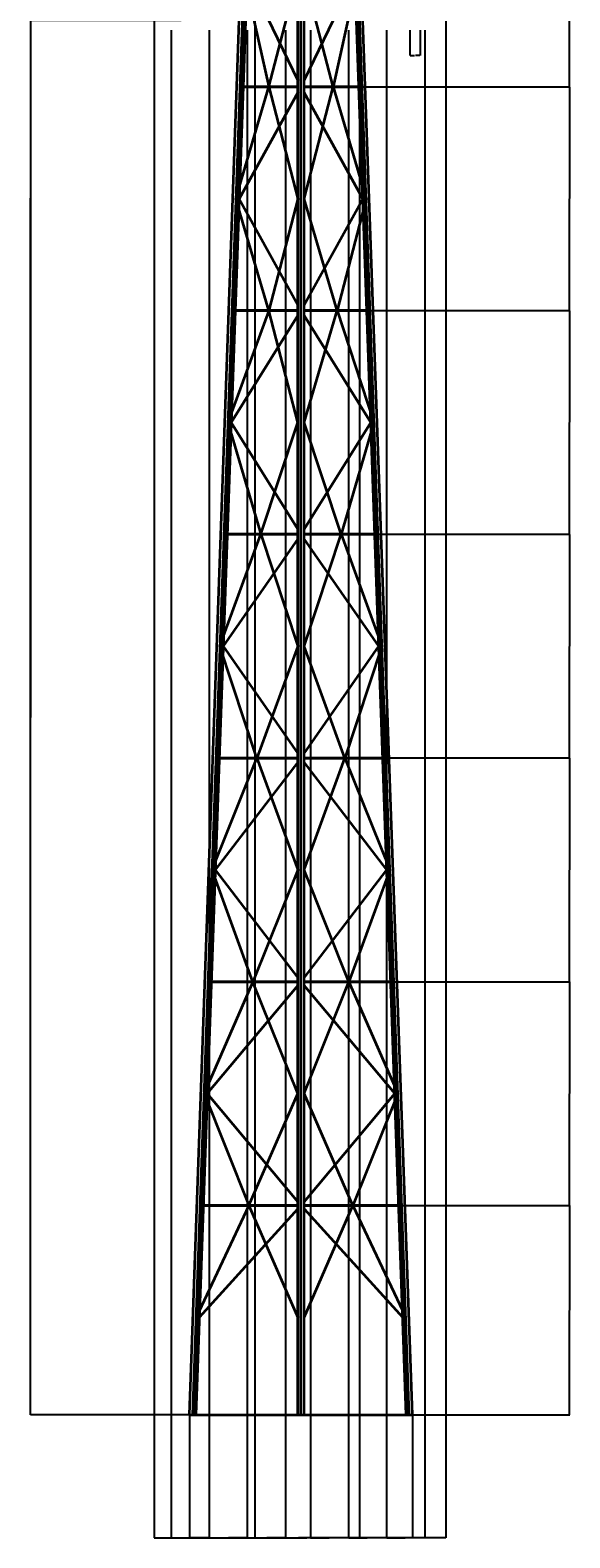
# Model space of a CAD drawing. Units: inches. Extents: x 3780 to 4301, y 1637 to 4224.
# Tile 1 of 8: x 3780 to 4301, y 1637 to 3092. Entities that reach past the tile are written whole.
import ezdxf

# ---------------------------------------------------------------- set-up
doc = ezdxf.new("R2010")
doc.units = ezdxf.units.IN
doc.layers.add('A-ANNO-DIMS', color=2, linetype='Continuous', lineweight=18)
doc.layers.add('S-TOWR', color=7, linetype='Continuous', lineweight=35)
doc.styles.get("Standard").update_dxf_attribs({"font": 'arial.ttf'})
doc.dimstyles.get("Standard").update_dxf_attribs({"dimtxt": 0.18, "dimasz": 0.18, "dimexe": 0.18, "dimexo": 0.0625, "dimgap": 0.09, "dimtad": 0, "dimtih": 1, "dimtoh": 1, "dimdec": 4, "dimzin": 0, "dimdsep": 46, "dimtxsty": 'Standard', "dimcen": 0.09, "dimadec": 0, "dimazin": 0, "dimtfac": 1, "dimtdec": 4, "dimtofl": 0, "dimtmove": 0, "dimatfit": 3, "dimfxl": 1, "dimtolj": 1, "dimtzin": 0, "dimarcsym": 0})

# ---------------------------------------------------------------- blocks, each defined once
blk = doc.blocks.new('*D10')
at = {"layer": 'A-ANNO-DIMS', "color": 0, "lineweight": -2, "transparency": 16777216}
for p, q in [((4146.7, 3092.2), (4146.7, 3067.7)), ((4156.5, 3092.2), (4156.5, 3067.7)), ((4146.9, 3067.9), (4151.1, 3067.9)), ((4156.3, 3067.9), (4152.1, 3067.9))]:
    blk.add_line(p, q, dxfattribs=at)
at = {"layer": 'A-ANNO-DIMS', "color": 0, "transparency": 16777216}
for points in [[(4146.9, 3067.9), (4146.9, 3067.9), (4146.7, 3067.9)], [(4156.3, 3067.9), (4156.3, 3067.9), (4156.5, 3067.9)]]:
    blk.add_solid(points, dxfattribs=at)
at = {"layer": 'Defpoints', "color": 0, "transparency": 16777216}
for p in [(4146.7, 3092.2), (4156.5, 3092.2), (4156.5, 3067.9)]:
    blk.add_point(p, dxfattribs=at)
at = {"layer": 'A-ANNO-DIMS', "color": 0, "transparency": 16777216, "insert": (4151.6, 3067.9), "char_height": 0.18, "attachment_point": 5}
blk.add_mtext('\\A1;10 TYP.', dxfattribs=at)
blk = doc.blocks.new('*D11')
at = {"layer": 'A-ANNO-DIMS', "color": 0, "lineweight": -2, "transparency": 16777216}
for p, q in [((3916.2, 4105.3), (3780.7, 4105.3)), ((3780.8, 4105.1), (3780.8, 2930.4)), ((3780.8, 1755.4), (3780.8, 2930.1)), ((3934.1, 1755.2), (3780.7, 1755.2))]:
    blk.add_line(p, q, dxfattribs=at)
at = {"layer": 'A-ANNO-DIMS', "color": 0, "transparency": 16777216}
for points in [[(3780.8, 4105.1), (3780.9, 4105.1), (3780.8, 4105.3)], [(3780.8, 1755.4), (3780.9, 1755.4), (3780.8, 1755.2)]]:
    blk.add_solid(points, dxfattribs=at)
at = {"layer": 'Defpoints', "color": 0, "transparency": 16777216}
for p in [(3780.8, 4105.3), (3916.3, 4105.3), (3934.2, 1755.2)]:
    blk.add_point(p, dxfattribs=at)
at = {"layer": 'A-ANNO-DIMS', "color": 0, "transparency": 16777216, "insert": (3780.8, 2930.3), "char_height": 0.18, "attachment_point": 5}
blk.add_mtext('\\A1;2350', dxfattribs=at)
blk = doc.blocks.new('*D12')
at = {"layer": 'A-ANNO-DIMS', "color": 0, "lineweight": -2, "transparency": 16777216}
for p, q in [((3934.2, 1755.2), (3934.2, 1636.6)), ((4149.2, 1755.2), (4149.2, 1636.6)), ((3934.3, 1636.7), (4041.4, 1636.7)), ((4149, 1636.7), (4042, 1636.7))]:
    blk.add_line(p, q, dxfattribs=at)
at = {"layer": 'A-ANNO-DIMS', "color": 0, "transparency": 16777216}
for points in [[(3934.3, 1636.8), (3934.3, 1636.7), (3934.2, 1636.7)], [(4149, 1636.8), (4149, 1636.7), (4149.2, 1636.7)]]:
    blk.add_solid(points, dxfattribs=at)
at = {"layer": 'Defpoints', "color": 0, "transparency": 16777216}
for p in [(3934.2, 1755.2), (4149.2, 1755.2), (4149.2, 1636.7)]:
    blk.add_point(p, dxfattribs=at)
at = {"layer": 'A-ANNO-DIMS', "color": 0, "transparency": 16777216, "insert": (4041.7, 1636.7), "char_height": 0.18, "attachment_point": 5}
blk.add_mtext('\\A1;215', dxfattribs=at)
blk = doc.blocks.new('*D13')
at = {"layer": 'A-ANNO-DIMS', "color": 0, "lineweight": -2, "transparency": 16777216}
for p, q in [((4044.7, 1957.5), (4300.9, 1957.5)), ((4300.7, 1957.3), (4300.7, 1856.5)), ((4300.7, 1755.4), (4300.7, 1856.2)), ((4044.7, 1755.2), (4300.9, 1755.2))]:
    blk.add_line(p, q, dxfattribs=at)
at = {"layer": 'A-ANNO-DIMS', "color": 0, "transparency": 16777216}
for points in [[(4300.7, 1957.3), (4300.7, 1957.3), (4300.7, 1957.5)], [(4300.7, 1755.4), (4300.7, 1755.4), (4300.7, 1755.2)]]:
    blk.add_solid(points, dxfattribs=at)
at = {"layer": 'Defpoints', "color": 0, "transparency": 16777216}
for p in [(4044.7, 1957.5), (4300.7, 1957.5), (4044.7, 1755.2)]:
    blk.add_point(p, dxfattribs=at)
at = {"layer": 'A-ANNO-DIMS', "color": 0, "transparency": 16777216, "insert": (4300.7, 1856.4), "char_height": 0.18, "attachment_point": 5}
blk.add_mtext('\\A1;202.2', dxfattribs=at)
blk = doc.blocks.new('*D14')
at = {"layer": 'A-ANNO-DIMS', "color": 0, "lineweight": -2, "transparency": 16777216}
for p, q in [((4044.7, 2173.5), (4300.9, 2173.5)), ((4300.7, 2173.3), (4300.7, 2065.6)), ((4300.7, 1957.6), (4300.7, 2065.3)), ((4044.7, 1957.5), (4300.9, 1957.5))]:
    blk.add_line(p, q, dxfattribs=at)
at = {"layer": 'A-ANNO-DIMS', "color": 0, "transparency": 16777216}
for points in [[(4300.7, 2173.3), (4300.7, 2173.3), (4300.7, 2173.5)], [(4300.7, 1957.6), (4300.7, 1957.6), (4300.7, 1957.5)]]:
    blk.add_solid(points, dxfattribs=at)
at = {"layer": 'Defpoints', "color": 0, "transparency": 16777216}
for p in [(4044.7, 2173.5), (4300.7, 2173.5), (4044.7, 1957.5)]:
    blk.add_point(p, dxfattribs=at)
at = {"layer": 'A-ANNO-DIMS', "color": 0, "transparency": 16777216, "insert": (4300.7, 2065.5), "char_height": 0.18, "attachment_point": 5}
blk.add_mtext('\\A1;216', dxfattribs=at)
blk = doc.blocks.new('*D15')
at = {"layer": 'A-ANNO-DIMS', "color": 0, "lineweight": -2, "transparency": 16777216}
for p, q in [((4044.7, 2389.5), (4300.9, 2389.5)), ((4300.7, 2389.3), (4300.7, 2281.6)), ((4300.7, 2173.6), (4300.7, 2281.3)), ((4044.7, 2173.5), (4300.9, 2173.5))]:
    blk.add_line(p, q, dxfattribs=at)
at = {"layer": 'A-ANNO-DIMS', "color": 0, "transparency": 16777216}
for points in [[(4300.7, 2389.3), (4300.7, 2389.3), (4300.7, 2389.5)], [(4300.7, 2173.6), (4300.7, 2173.6), (4300.7, 2173.5)]]:
    blk.add_solid(points, dxfattribs=at)
at = {"layer": 'Defpoints', "color": 0, "transparency": 16777216}
for p in [(4044.7, 2389.5), (4300.7, 2389.5), (4044.7, 2173.5)]:
    blk.add_point(p, dxfattribs=at)
at = {"layer": 'A-ANNO-DIMS', "color": 0, "transparency": 16777216, "insert": (4300.7, 2281.5), "char_height": 0.18, "attachment_point": 5}
blk.add_mtext('\\A1;216', dxfattribs=at)
blk = doc.blocks.new('*D16')
at = {"layer": 'A-ANNO-DIMS', "color": 0, "lineweight": -2, "transparency": 16777216}
for p, q in [((4044.7, 2605.5), (4300.9, 2605.5)), ((4300.7, 2605.3), (4300.7, 2497.6)), ((4300.7, 2389.6), (4300.7, 2497.3)), ((4044.7, 2389.5), (4300.9, 2389.5))]:
    blk.add_line(p, q, dxfattribs=at)
at = {"layer": 'A-ANNO-DIMS', "color": 0, "transparency": 16777216}
for points in [[(4300.7, 2605.3), (4300.7, 2605.3), (4300.7, 2605.5)], [(4300.7, 2389.6), (4300.7, 2389.6), (4300.7, 2389.5)]]:
    blk.add_solid(points, dxfattribs=at)
at = {"layer": 'Defpoints', "color": 0, "transparency": 16777216}
for p in [(4044.7, 2605.5), (4300.7, 2605.5), (4044.7, 2389.5)]:
    blk.add_point(p, dxfattribs=at)
at = {"layer": 'A-ANNO-DIMS', "color": 0, "transparency": 16777216, "insert": (4300.7, 2497.5), "char_height": 0.18, "attachment_point": 5}
blk.add_mtext('\\A1;216', dxfattribs=at)
blk = doc.blocks.new('*D17')
at = {"layer": 'A-ANNO-DIMS', "color": 0, "lineweight": -2, "transparency": 16777216}
for p, q in [((4044.7, 2821.5), (4300.9, 2821.5)), ((4300.7, 2821.3), (4300.7, 2713.6)), ((4300.7, 2605.6), (4300.7, 2713.3)), ((4044.7, 2605.5), (4300.9, 2605.5))]:
    blk.add_line(p, q, dxfattribs=at)
at = {"layer": 'A-ANNO-DIMS', "color": 0, "transparency": 16777216}
for points in [[(4300.7, 2821.3), (4300.7, 2821.3), (4300.7, 2821.5)], [(4300.7, 2605.6), (4300.7, 2605.6), (4300.7, 2605.5)]]:
    blk.add_solid(points, dxfattribs=at)
at = {"layer": 'Defpoints', "color": 0, "transparency": 16777216}
for p in [(4044.7, 2821.5), (4300.7, 2821.5), (4044.7, 2605.5)]:
    blk.add_point(p, dxfattribs=at)
at = {"layer": 'A-ANNO-DIMS', "color": 0, "transparency": 16777216, "insert": (4300.7, 2713.5), "char_height": 0.18, "attachment_point": 5}
blk.add_mtext('\\A1;216', dxfattribs=at)
blk = doc.blocks.new('*D18')
at = {"layer": 'A-ANNO-DIMS', "color": 0, "lineweight": -2, "transparency": 16777216}
for p, q in [((4044.7, 3037.5), (4300.9, 3037.5)), ((4300.7, 3037.3), (4300.7, 2929.6)), ((4300.7, 2821.6), (4300.7, 2929.3)), ((4044.7, 2821.5), (4300.9, 2821.5))]:
    blk.add_line(p, q, dxfattribs=at)
at = {"layer": 'A-ANNO-DIMS', "color": 0, "transparency": 16777216}
for points in [[(4300.7, 3037.3), (4300.7, 3037.3), (4300.7, 3037.5)], [(4300.7, 2821.6), (4300.7, 2821.6), (4300.7, 2821.5)]]:
    blk.add_solid(points, dxfattribs=at)
at = {"layer": 'Defpoints', "color": 0, "transparency": 16777216}
for p in [(4044.7, 3037.5), (4300.7, 3037.5), (4044.7, 2821.5)]:
    blk.add_point(p, dxfattribs=at)
at = {"layer": 'A-ANNO-DIMS', "color": 0, "transparency": 16777216, "insert": (4300.7, 2929.5), "char_height": 0.18, "attachment_point": 5}
blk.add_mtext('\\A1;216', dxfattribs=at)
blk = doc.blocks.new('*D19')
at = {"layer": 'A-ANNO-DIMS', "color": 0, "lineweight": -2, "transparency": 16777216}
for p, q in [((4044.7, 3253.5), (4300.9, 3253.5)), ((4300.7, 3253.3), (4300.7, 3145.6)), ((4300.7, 3037.6), (4300.7, 3145.3)), ((4044.7, 3037.5), (4300.9, 3037.5))]:
    blk.add_line(p, q, dxfattribs=at)
at = {"layer": 'A-ANNO-DIMS', "color": 0, "transparency": 16777216}
for points in [[(4300.7, 3253.3), (4300.7, 3253.3), (4300.7, 3253.5)], [(4300.7, 3037.6), (4300.7, 3037.6), (4300.7, 3037.5)]]:
    blk.add_solid(points, dxfattribs=at)
at = {"layer": 'Defpoints', "color": 0, "transparency": 16777216}
for p in [(4044.7, 3253.5), (4300.7, 3253.5), (4044.7, 3037.5)]:
    blk.add_point(p, dxfattribs=at)
at = {"layer": 'A-ANNO-DIMS', "color": 0, "transparency": 16777216, "insert": (4300.7, 3145.5), "char_height": 0.18, "attachment_point": 5}
blk.add_mtext('\\A1;216', dxfattribs=at)
blk = doc.blocks.new('*D22')
at = {"layer": 'A-ANNO-DIMS', "color": 0, "lineweight": -2, "transparency": 16777216}
for p, q in [((3900, 3694), (3900, 1636.6)), ((4181.5, 3694), (4181.5, 1636.6)), ((3900.2, 1636.7), (4040.3, 1636.7)), ((4181.3, 1636.7), (4041.2, 1636.7))]:
    blk.add_line(p, q, dxfattribs=at)
at = {"layer": 'A-ANNO-DIMS', "color": 0, "transparency": 16777216}
for points in [[(3900.2, 1636.8), (3900.2, 1636.7), (3900, 1636.7)], [(4181.3, 1636.8), (4181.3, 1636.7), (4181.5, 1636.7)]]:
    blk.add_solid(points, dxfattribs=at)
at = {"layer": 'Defpoints', "color": 0, "transparency": 16777216}
for p in [(3900, 3694.1), (4181.5, 3694.1), (4181.5, 1636.7)]:
    blk.add_point(p, dxfattribs=at)
at = {"layer": 'A-ANNO-DIMS', "color": 0, "transparency": 16777216, "insert": (4040.8, 1636.7), "char_height": 0.18, "attachment_point": 5}
blk.add_mtext('\\A1;281.45', dxfattribs=at)
blk = doc.blocks.new('*D26')
at = {"layer": 'A-ANNO-DIMS', "color": 0, "lineweight": -2, "transparency": 16777216}
for p, q in [((3926.2, 3101.6), (3780.7, 3101.6)), ((3780.8, 3101.4), (3780.8, 2428.6)), ((3780.8, 1755.4), (3780.8, 2428.2)), ((3934.1, 1755.2), (3780.7, 1755.2))]:
    blk.add_line(p, q, dxfattribs=at)
at = {"layer": 'A-ANNO-DIMS', "color": 0, "transparency": 16777216}
for points in [[(3780.8, 3101.4), (3780.9, 3101.4), (3780.8, 3101.6)], [(3780.8, 1755.4), (3780.9, 1755.4), (3780.8, 1755.2)]]:
    blk.add_solid(points, dxfattribs=at)
at = {"layer": 'Defpoints', "color": 0, "transparency": 16777216}
for p in [(3780.8, 3101.6), (3926.2, 3101.6), (3934.2, 1755.2)]:
    blk.add_point(p, dxfattribs=at)
at = {"layer": 'A-ANNO-DIMS', "color": 0, "transparency": 16777216, "insert": (3780.8, 2428.4), "char_height": 0.18, "attachment_point": 5}
blk.add_mtext('\\A1;1346.3', dxfattribs=at)
blk = doc.blocks.new('*D42')
at = {"layer": 'A-ANNO-DIMS', "color": 0, "lineweight": -2, "transparency": 16777216}
for p, q in [((3997.1, 3538.4), (3997.1, 1636.6)), ((4098.1, 3539.6), (4098.1, 1636.6)), ((3997.3, 1636.7), (4047.4, 1636.7)), ((4098, 1636.7), (4047.9, 1636.7))]:
    blk.add_line(p, q, dxfattribs=at)
at = {"layer": 'A-ANNO-DIMS', "color": 0, "transparency": 16777216}
for points in [[(3997.3, 1636.8), (3997.3, 1636.7), (3997.1, 1636.7)], [(4098, 1636.8), (4098, 1636.7), (4098.1, 1636.7)]]:
    blk.add_solid(points, dxfattribs=at)
at = {"layer": 'Defpoints', "color": 0, "transparency": 16777216}
for p in [(3997.1, 3538.5), (4098.1, 3539.7), (4098.1, 1636.7)]:
    blk.add_point(p, dxfattribs=at)
at = {"layer": 'A-ANNO-DIMS', "color": 0, "transparency": 16777216, "insert": (4047.6, 1636.7), "char_height": 0.18, "attachment_point": 5}
blk.add_mtext('\\A1;101', dxfattribs=at)
blk = doc.blocks.new('*D51')
at = {"layer": 'A-ANNO-DIMS', "color": 0, "lineweight": -2, "transparency": 16777216}
for p, q in [((3916.4, 3092.2), (3916.4, 1636.6)), ((3953.1, 3092.2), (3953.1, 1636.6)), ((3916.6, 1636.7), (3934.4, 1636.7)), ((3953, 1636.7), (3935.2, 1636.7))]:
    blk.add_line(p, q, dxfattribs=at)
at = {"layer": 'A-ANNO-DIMS', "color": 0, "transparency": 16777216}
for points in [[(3916.6, 1636.8), (3916.6, 1636.7), (3916.4, 1636.7)], [(3953, 1636.8), (3953, 1636.7), (3953.1, 1636.7)]]:
    blk.add_solid(points, dxfattribs=at)
at = {"layer": 'Defpoints', "color": 0, "transparency": 16777216}
for p in [(3916.4, 3092.2), (3953.1, 3092.2), (3953.1, 1636.7)]:
    blk.add_point(p, dxfattribs=at)
at = {"layer": 'A-ANNO-DIMS', "color": 0, "transparency": 16777216, "insert": (3934.8, 1636.7), "char_height": 0.18, "attachment_point": 5}
blk.add_mtext('\\A1;36.75', dxfattribs=at)
blk = doc.blocks.new('*D52')
at = {"layer": 'A-ANNO-DIMS', "color": 0, "lineweight": -2, "transparency": 16777216}
for p, q in [((3953.1, 3092.2), (3953.1, 1636.6)), ((3989.9, 3092.2), (3989.9, 1636.6)), ((3953.3, 1636.7), (3971.1, 1636.7)), ((3989.7, 1636.7), (3971.9, 1636.7))]:
    blk.add_line(p, q, dxfattribs=at)
at = {"layer": 'A-ANNO-DIMS', "color": 0, "transparency": 16777216}
for points in [[(3953.3, 1636.8), (3953.3, 1636.7), (3953.1, 1636.7)], [(3989.7, 1636.8), (3989.7, 1636.7), (3989.9, 1636.7)]]:
    blk.add_solid(points, dxfattribs=at)
at = {"layer": 'Defpoints', "color": 0, "transparency": 16777216}
for p in [(3953.1, 3092.2), (3989.9, 3092.2), (3989.9, 1636.7)]:
    blk.add_point(p, dxfattribs=at)
at = {"layer": 'A-ANNO-DIMS', "color": 0, "transparency": 16777216, "insert": (3971.5, 1636.7), "char_height": 0.18, "attachment_point": 5}
blk.add_mtext('\\A1;36.75', dxfattribs=at)
blk = doc.blocks.new('*D53')
at = {"layer": 'A-ANNO-DIMS', "color": 0, "lineweight": -2, "transparency": 16777216}
for p, q in [((3989.9, 3092.2), (3989.9, 1636.6)), ((4026.6, 3092.2), (4026.6, 1636.6)), ((3990.1, 1636.7), (4007.9, 1636.7)), ((4026.5, 1636.7), (4008.7, 1636.7))]:
    blk.add_line(p, q, dxfattribs=at)
at = {"layer": 'A-ANNO-DIMS', "color": 0, "transparency": 16777216}
for points in [[(3990.1, 1636.8), (3990.1, 1636.7), (3989.9, 1636.7)], [(4026.5, 1636.8), (4026.5, 1636.7), (4026.6, 1636.7)]]:
    blk.add_solid(points, dxfattribs=at)
at = {"layer": 'Defpoints', "color": 0, "transparency": 16777216}
for p in [(3989.9, 3092.2), (4026.6, 3092.2), (4026.6, 1636.7)]:
    blk.add_point(p, dxfattribs=at)
at = {"layer": 'A-ANNO-DIMS', "color": 0, "transparency": 16777216, "insert": (4008.3, 1636.7), "char_height": 0.18, "attachment_point": 5}
blk.add_mtext('\\A1;36.75', dxfattribs=at)
blk = doc.blocks.new('*D54')
at = {"layer": 'A-ANNO-DIMS', "color": 0, "lineweight": -2, "transparency": 16777216}
for p, q in [((4026.6, 3092.2), (4026.6, 1636.6)), ((4050.8, 3092.2), (4050.8, 1636.6)), ((4026.8, 1636.7), (4038.3, 1636.7)), ((4050.6, 1636.7), (4039.2, 1636.7))]:
    blk.add_line(p, q, dxfattribs=at)
at = {"layer": 'A-ANNO-DIMS', "color": 0, "transparency": 16777216}
for points in [[(4026.8, 1636.8), (4026.8, 1636.7), (4026.6, 1636.7)], [(4050.6, 1636.8), (4050.6, 1636.7), (4050.8, 1636.7)]]:
    blk.add_solid(points, dxfattribs=at)
at = {"layer": 'Defpoints', "color": 0, "transparency": 16777216}
for p in [(4026.6, 3092.2), (4050.8, 3092.2), (4050.8, 1636.7)]:
    blk.add_point(p, dxfattribs=at)
at = {"layer": 'A-ANNO-DIMS', "color": 0, "transparency": 16777216, "insert": (4038.7, 1636.7), "char_height": 0.18, "attachment_point": 5}
blk.add_mtext('\\A1;24.147', dxfattribs=at)
blk = doc.blocks.new('*D55')
at = {"layer": 'A-ANNO-DIMS', "color": 0, "lineweight": -2, "transparency": 16777216}
for p, q in [((4050.8, 3092.2), (4050.8, 1636.6)), ((4087.5, 3092.2), (4087.5, 1636.6)), ((4051, 1636.7), (4068.8, 1636.7)), ((4087.4, 1636.7), (4069.6, 1636.7))]:
    blk.add_line(p, q, dxfattribs=at)
at = {"layer": 'A-ANNO-DIMS', "color": 0, "transparency": 16777216}
for points in [[(4051, 1636.8), (4051, 1636.7), (4050.8, 1636.7)], [(4087.4, 1636.8), (4087.4, 1636.7), (4087.5, 1636.7)]]:
    blk.add_solid(points, dxfattribs=at)
at = {"layer": 'Defpoints', "color": 0, "transparency": 16777216}
for p in [(4050.8, 3092.2), (4087.5, 3092.2), (4087.5, 1636.7)]:
    blk.add_point(p, dxfattribs=at)
at = {"layer": 'A-ANNO-DIMS', "color": 0, "transparency": 16777216, "insert": (4069.2, 1636.7), "char_height": 0.18, "attachment_point": 5}
blk.add_mtext('\\A1;36.75', dxfattribs=at)
blk = doc.blocks.new('*D56')
at = {"layer": 'A-ANNO-DIMS', "color": 0, "lineweight": -2, "transparency": 16777216}
for p, q in [((4087.5, 3092.2), (4087.5, 1636.6)), ((4124.3, 3092.2), (4124.3, 1636.6)), ((4087.7, 1636.7), (4105.5, 1636.7)), ((4124.1, 1636.7), (4106.3, 1636.7))]:
    blk.add_line(p, q, dxfattribs=at)
at = {"layer": 'A-ANNO-DIMS', "color": 0, "transparency": 16777216}
for points in [[(4087.7, 1636.8), (4087.7, 1636.7), (4087.5, 1636.7)], [(4124.1, 1636.8), (4124.1, 1636.7), (4124.3, 1636.7)]]:
    blk.add_solid(points, dxfattribs=at)
at = {"layer": 'Defpoints', "color": 0, "transparency": 16777216}
for p in [(4087.5, 3092.2), (4124.3, 3092.2), (4124.3, 1636.7)]:
    blk.add_point(p, dxfattribs=at)
at = {"layer": 'A-ANNO-DIMS', "color": 0, "transparency": 16777216, "insert": (4105.9, 1636.7), "char_height": 0.18, "attachment_point": 5}
blk.add_mtext('\\A1;36.75', dxfattribs=at)
blk = doc.blocks.new('*D57')
at = {"layer": 'A-ANNO-DIMS', "color": 0, "lineweight": -2, "transparency": 16777216}
for p, q in [((4124.3, 3092.2), (4124.3, 1636.6)), ((4161, 3092.2), (4161, 1636.6)), ((4124.5, 1636.7), (4142.3, 1636.7)), ((4160.9, 1636.7), (4143.1, 1636.7))]:
    blk.add_line(p, q, dxfattribs=at)
at = {"layer": 'A-ANNO-DIMS', "color": 0, "transparency": 16777216}
for points in [[(4124.5, 1636.8), (4124.5, 1636.7), (4124.3, 1636.7)], [(4160.9, 1636.8), (4160.9, 1636.7), (4161, 1636.7)]]:
    blk.add_solid(points, dxfattribs=at)
at = {"layer": 'Defpoints', "color": 0, "transparency": 16777216}
for p in [(4124.3, 3092.2), (4161, 3092.2), (4161, 1636.7)]:
    blk.add_point(p, dxfattribs=at)
at = {"layer": 'A-ANNO-DIMS', "color": 0, "transparency": 16777216, "insert": (4142.7, 1636.7), "char_height": 0.18, "attachment_point": 5}
blk.add_mtext('\\A1;36.75', dxfattribs=at)

msp = doc.modelspace()

# ---------------------------------------------------------------- linework, layer by layer
at = {"layer": 'S-TOWR'}
for p, q in [((3987.2641, 3164.2144), (3937.1525, 1755.2487)), ((3938.4515, 1755.2487), (3988.5631, 3164.2144)), ((4038.6622, 1755.2487), (4038.6622, 3161.2144)), ((4041.6622, 1755.2487), (4041.6622, 3164.2144)), ((4044.6622, 1755.2487), (4044.6622, 3161.2144)), ((4144.8729, 1755.2487), (4094.7613, 3164.2144)), ((4146.1719, 1755.2487), (4096.0603, 3164.2144)), ((3986.5972, 3145.4644), (4010.7091, 3037.4644)), ((4010.7091, 3037.4644), (4038.6622, 3145.4644)), ((4072.6153, 3037.4644), (4044.6622, 3145.4644)), ((4096.7272, 3145.4644), (4072.6153, 3037.4644)), ((3934.1525, 1755.2487), (3982.0358, 3101.5639)), ((3988.3368, 3110.0269), (3940.1525, 1755.2487)), ((4009.4815, 3104.2179), (4038.6622, 3043.6874)), ((4044.6622, 3043.6874), (4073.2315, 3102.9495)), ((4143.1719, 1755.2487), (4095.2886, 3101.5639)), ((4149.1719, 1755.2487), (4101.2886, 3101.5639)), ((3978.9149, 2929.4644), (4010.7091, 3037.4644)), ((4038.6622, 3032.0416), (3981.9149, 2929.4644)), ((3982.756, 3037.4644), (4010.7091, 3037.4644)), ((4038.6622, 3037.4644), (3985.756, 3037.4644)), ((4010.7091, 3037.4644), (4038.6622, 3037.4644)), ((4010.7091, 3037.4644), (4038.6622, 2929.4644)), ((4097.5683, 3037.4644), (4044.6622, 3037.4644)), ((4044.6622, 3037.4644), (4072.6153, 3037.4644)), ((4044.6622, 2929.4644), (4072.6153, 3037.4644)), ((4101.4095, 2929.4644), (4044.6622, 3032.0416)), ((4072.6153, 3037.4644), (4100.5683, 3037.4644)), ((4072.6153, 3037.4644), (4104.4095, 2929.4644)), ((4010.7091, 2821.4644), (3978.9149, 2929.4644)), ((3981.9149, 2929.4644), (4038.6622, 2826.8873)), ((4038.6622, 2929.4644), (4010.7091, 2821.4644)), ((4044.6622, 2826.8873), (4101.4095, 2929.4644)), ((4076.4564, 2821.4644), (4044.6622, 2929.4644)), ((4104.4095, 2929.4644), (4076.4564, 2821.4644)), ((4010.7091, 2821.4644), (3971.2326, 2713.4644)), ((4038.6622, 2816.6594), (3974.2326, 2713.4644)), ((3975.0737, 2821.4644), (4010.7091, 2821.4644)), ((4038.6622, 2821.4644), (3978.0737, 2821.4644)), ((4010.7091, 2821.4644), (4038.6622, 2821.4644)), ((4038.6622, 2713.4644), (4010.7091, 2821.4644)), ((4105.2507, 2821.4644), (4044.6622, 2821.4644)), ((4044.6622, 2821.4644), (4076.4564, 2821.4644)), ((4044.6622, 2713.4644), (4076.4564, 2821.4644)), ((4109.0918, 2713.4644), (4044.6622, 2816.6594)), ((4076.4564, 2821.4644), (4108.2507, 2821.4644)), ((4076.4564, 2821.4644), (4112.0918, 2713.4644)), ((3971.2326, 2713.4644), (4003.0268, 2605.4644)), ((3974.2326, 2713.4644), (4038.6622, 2610.2694)), ((4003.0268, 2605.4644), (4038.6622, 2713.4644)), ((4044.6622, 2610.2694), (4109.0918, 2713.4644)), ((4080.2976, 2605.4644), (4044.6622, 2713.4644)), ((4112.0918, 2713.4644), (4080.2976, 2605.4644)), ((3963.5503, 2497.4644), (4003.0268, 2605.4644)), ((4038.6622, 2601.1509), (3966.5503, 2497.4644)), ((3967.3914, 2605.4644), (4003.0268, 2605.4644)), ((4038.6622, 2605.4644), (3970.3914, 2605.4644)), ((4003.0268, 2605.4644), (4038.6622, 2605.4644)), ((4003.0268, 2605.4644), (4038.6622, 2497.4644)), ((4044.6622, 2605.4644), (4080.2976, 2605.4644)), ((4112.933, 2605.4644), (4044.6622, 2605.4644)), ((4044.6622, 2497.4644), (4080.2976, 2605.4644)), ((4116.7741, 2497.4644), (4044.6622, 2601.1509)), ((4080.2976, 2605.4644), (4115.933, 2605.4644)), ((4080.2976, 2605.4644), (4119.7741, 2497.4644)), ((3999.1857, 2389.4644), (3963.5503, 2497.4644)), ((3966.5503, 2497.4644), (4038.6622, 2393.778)), ((4038.6622, 2497.4644), (3999.1857, 2389.4644)), ((4044.6622, 2393.778), (4116.7741, 2497.4644)), ((4084.1387, 2389.4644), (4044.6622, 2497.4644)), ((4119.7741, 2497.4644), (4084.1387, 2389.4644)), ((3955.868, 2281.4644), (3999.1857, 2389.4644)), ((3959.7091, 2389.4644), (3999.1857, 2389.4644)), ((4038.6622, 2389.4644), (3962.7091, 2389.4644)), ((3999.1857, 2389.4644), (4038.6622, 2389.4644)), ((3999.1857, 2389.4644), (4038.6622, 2281.4644)), ((4120.6153, 2389.4644), (4044.6622, 2389.4644)), ((4044.6622, 2389.4644), (4084.1387, 2389.4644)), ((4044.6622, 2281.4644), (4084.1387, 2389.4644)), ((4084.1387, 2389.4644), (4123.6153, 2389.4644)), ((4084.1387, 2389.4644), (4127.4564, 2281.4644)), ((4038.6622, 2385.5511), (3958.868, 2281.4644)), ((4124.4564, 2281.4644), (4044.6622, 2385.5511)), ((3995.3445, 2173.4644), (3955.868, 2281.4644)), ((3958.868, 2281.4644), (4038.6622, 2177.3777)), ((4038.6622, 2281.4644), (3995.3445, 2173.4644)), ((4044.6622, 2177.3777), (4124.4564, 2281.4644)), ((4087.9799, 2173.4644), (4044.6622, 2281.4644)), ((4127.4564, 2281.4644), (4087.9799, 2173.4644)), ((3995.3445, 2173.4644), (3948.1857, 2065.4644)), ((4038.6622, 2169.8834), (3951.1857, 2065.4644)), ((3952.0268, 2173.4644), (3995.3445, 2173.4644)), ((4038.6622, 2173.4644), (3955.0268, 2173.4644)), ((3995.3445, 2173.4644), (4038.6622, 2173.4644)), ((4038.6622, 2065.4644), (3995.3445, 2173.4644)), ((4128.2976, 2173.4644), (4044.6622, 2173.4644)), ((4044.6622, 2173.4644), (4087.9799, 2173.4644)), ((4044.6622, 2065.4644), (4087.9799, 2173.4644)), ((4132.1387, 2065.4644), (4044.6622, 2169.8834)), ((4087.9799, 2173.4644), (4131.2976, 2173.4644)), ((4087.9799, 2173.4644), (4135.1387, 2065.4644)), ((3948.1857, 2065.4644), (3991.5034, 1957.4644)), ((3951.1857, 2065.4644), (4038.6622, 1961.0455)), ((3991.5034, 1957.4644), (4038.6622, 2065.4644)), ((4044.6622, 1961.0455), (4132.1387, 2065.4644)), ((4091.821, 1957.4644), (4044.6622, 2065.4644)), ((4135.1387, 2065.4644), (4091.821, 1957.4644)), ((3991.5034, 1957.4644), (3940.5034, 1849.4644)), ((4038.6622, 1954.1636), (3943.5034, 1849.4644)), ((3944.3445, 1957.4644), (3991.5034, 1957.4644)), ((4038.6622, 1957.4644), (3947.3445, 1957.4644)), ((3991.5034, 1957.4644), (4038.6622, 1957.4644)), ((3991.5034, 1957.4644), (4038.6622, 1849.4644)), ((4044.6622, 1957.4644), (4091.821, 1957.4644)), ((4135.9799, 1957.4644), (4044.6622, 1957.4644)), ((4044.6622, 1849.4644), (4091.821, 1957.4644)), ((4044.6622, 1954.1636), (4139.821, 1849.4644)), ((4091.821, 1957.4644), (4138.9799, 1957.4644)), ((4091.821, 1957.4644), (4142.821, 1849.4644)), ((4144.5542, 1764.2104), (4144.5524, 1764.2596)), ((3934.1525, 1755.2487), (4149.1719, 1755.2487)), ((3938.4548, 1755.3411), (3938.4566, 1755.391))]:
    msp.add_line(p, q, dxfattribs=at)

# ---------------------------------------------------------------- dimensions: what is measured, and where the dimension line sits
at = {"layer": 'A-ANNO-DIMS'}
for base, p1, p2, override, picture, middle in [((3780.8371, 4105.2769), (3934.1525, 1755.2487), (3916.252, 4105.2769), {"dimdec": 0, "dimlfac": 1, "dimrnd": 0, "dimzin": 0, "dimdsep": 46, "dimlunit": 2}, '*D11', (3780.8371, 2930.2628)), ((4300.7091, 3253.4644), (4044.6622, 3037.4644), (4044.6622, 3253.4644), {"dimdec": 0, "dimlfac": 1, "dimrnd": 0, "dimzin": 0, "dimdsep": 46, "dimlunit": 2}, '*D19', (4300.7091, 3145.4644)), ((3780.8371, 3101.5639), (3934.1525, 1755.2487), (3926.2315, 3101.5639), {"dimdec": 1, "dimlfac": 1, "dimrnd": 0, "dimzin": 0, "dimdsep": 46, "dimlunit": 2}, '*D26', (3780.8371, 2428.4063)), ((4300.7091, 3037.4644), (4044.6622, 2821.4644), (4044.6622, 3037.4644), {"dimdec": 0, "dimlfac": 1, "dimrnd": 0, "dimzin": 0, "dimdsep": 46, "dimlunit": 2}, '*D18', (4300.7091, 2929.4644)), ((4300.7091, 2821.4644), (4044.6622, 2605.4644), (4044.6622, 2821.4644), {"dimdec": 0, "dimlfac": 1, "dimrnd": 0, "dimzin": 0, "dimdsep": 46, "dimlunit": 2}, '*D17', (4300.7091, 2713.4644)), ((4300.7091, 2605.4644), (4044.6622, 2389.4644), (4044.6622, 2605.4644), {"dimdec": 0, "dimlfac": 1, "dimrnd": 0, "dimzin": 0, "dimdsep": 46, "dimlunit": 2}, '*D16', (4300.7091, 2497.4644)), ((4300.7091, 2389.4644), (4044.6622, 2173.4644), (4044.6622, 2389.4644), {"dimdec": 0, "dimlfac": 1, "dimrnd": 0, "dimzin": 0, "dimdsep": 46, "dimlunit": 2}, '*D15', (4300.7091, 2281.4644)), ((4300.7091, 2173.4644), (4044.6622, 1957.4644), (4044.6622, 2173.4644), {"dimdec": 0, "dimlfac": 1, "dimrnd": 0, "dimzin": 0, "dimdsep": 46, "dimlunit": 2}, '*D14', (4300.7091, 2065.4644)), ((4300.7091, 1957.4644), (4044.6622, 1755.2487), (4044.6622, 1957.4644), {"dimdec": 1, "dimlfac": 1, "dimrnd": 0, "dimzin": 0, "dimdsep": 46, "dimlunit": 2}, '*D13', (4300.7091, 1856.3566))]:
    dim = msp.add_linear_dim(base=base, p1=p1, p2=p2, angle=90, dimstyle='Standard', override=override, dxfattribs=at)
    dim.commit()
    dim.dimension.update_dxf_attribs({"geometry": picture, "text_midpoint": middle})
for base, p1, p2, override, picture, middle in [((4181.498, 1636.7487), (3900.0482, 3694.0677), (4181.498, 3694.0677), {"dimdec": 2, "dimlfac": 1, "dimrnd": 0, "dimzin": 0, "dimdsep": 46, "dimlunit": 2}, '*D22', (4040.7731, 1636.7487)), ((4098.1498, 1636.7487), (3997.1451, 3538.4672), (4098.1498, 3539.6986), {"dimdec": 0, "dimlfac": 1, "dimrnd": 0, "dimzin": 0, "dimdsep": 46, "dimlunit": 2}, '*D42', (4047.6474, 1636.7487)), ((3953.144, 1636.7487), (3916.394, 3092.2144), (3953.144, 3092.2144), {"dimdec": 2, "dimlfac": 1, "dimrnd": 0, "dimzin": 0, "dimdsep": 46, "dimlunit": 2}, '*D51', (3934.769, 1636.7487)), ((3989.894, 1636.7487), (3953.144, 3092.2144), (3989.894, 3092.2144), {"dimdec": 2, "dimlfac": 1, "dimrnd": 0, "dimzin": 0, "dimdsep": 46, "dimlunit": 2}, '*D52', (3971.519, 1636.7487)), ((4026.644, 1636.7487), (3989.894, 3092.2144), (4026.644, 3092.2144), {"dimdec": 2, "dimlfac": 1, "dimrnd": 0, "dimzin": 0, "dimdsep": 46, "dimlunit": 2}, '*D53', (4008.269, 1636.7487)), ((4050.7911, 1636.7487), (4026.644, 3092.2144), (4050.7911, 3092.2144), {"dimdec": 3, "dimlfac": 1, "dimrnd": 0, "dimzin": 0, "dimdsep": 46, "dimlunit": 2}, '*D54', (4038.7176, 1636.7487)), ((4087.5411, 1636.7487), (4050.7911, 3092.2144), (4087.5411, 3092.2144), {"dimdec": 2, "dimlfac": 1, "dimrnd": 0, "dimzin": 0, "dimdsep": 46, "dimlunit": 2}, '*D55', (4069.1661, 1636.7487)), ((4124.2911, 1636.7487), (4087.5411, 3092.2144), (4124.2911, 3092.2144), {"dimdec": 2, "dimlfac": 1, "dimrnd": 0, "dimzin": 0, "dimdsep": 46, "dimlunit": 2}, '*D56', (4105.9161, 1636.7487)), ((4161.0411, 1636.7487), (4124.2911, 3092.2144), (4161.0411, 3092.2144), {"dimdec": 2, "dimlfac": 1, "dimrnd": 0, "dimzin": 0, "dimdsep": 46, "dimlunit": 2}, '*D57', (4142.6661, 1636.7487)), ((4149.1719, 1636.7487), (3934.1525, 1755.2487), (4149.1719, 1755.2487), {"dimdec": 0, "dimlfac": 1, "dimrnd": 0, "dimzin": 0, "dimdsep": 46, "dimlunit": 2}, '*D12', (4041.6622, 1636.7487))]:
    dim = msp.add_linear_dim(base=base, p1=p1, p2=p2, dimstyle='Standard', override=override, dxfattribs=at)
    dim.commit()
    dim.dimension.update_dxf_attribs({"geometry": picture, "text_midpoint": middle})
dim = msp.add_linear_dim(base=(4156.4815, 3067.9144), p1=(4146.7315, 3092.2144), p2=(4156.4815, 3092.2144), text='<> TYP.', dimstyle='Standard', override={"dimdec": 0, "dimlfac": 1, "dimrnd": 0, "dimzin": 0, "dimdsep": 46, "dimlunit": 2}, dxfattribs=at)
dim.commit()
dim.dimension.update_dxf_attribs({"geometry": '*D10', "text_midpoint": (4151.6065, 3067.9144)})

doc.saveas('drawing.dxf')
